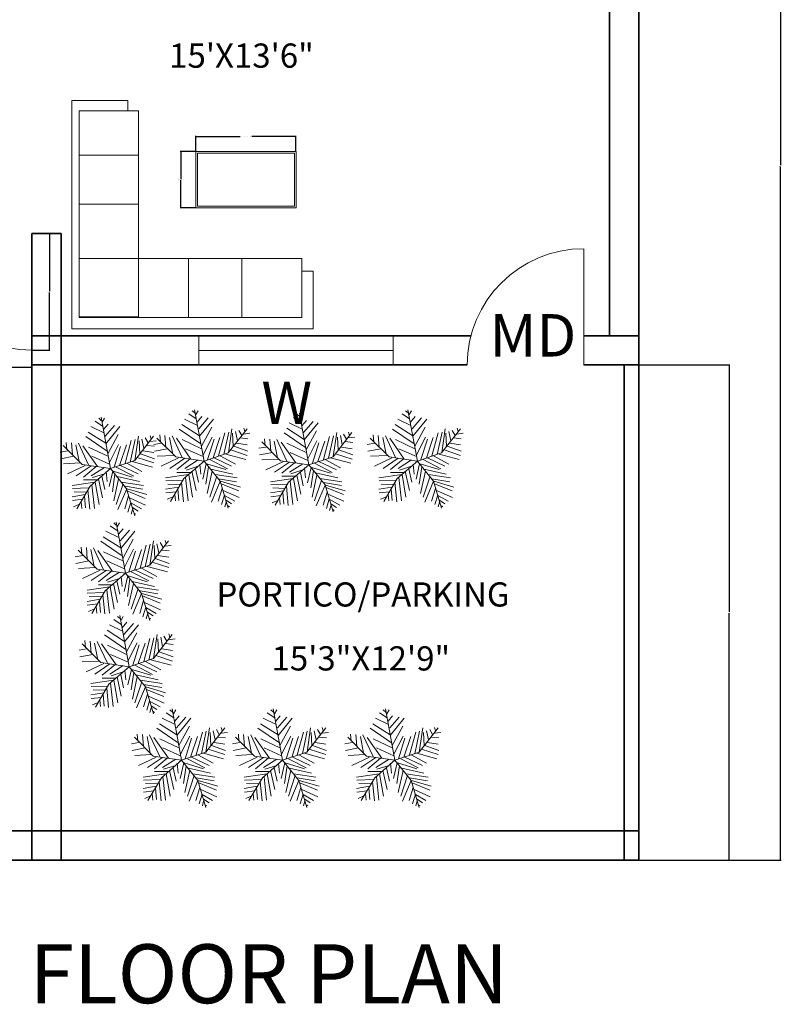
# Model space of a CAD drawing. Units: inches. Extents: x -26 to 788, y -42 to 505.
# Tile 4 of 9: x 116 to 352, y -42 to 262. Entities that reach past the tile are written whole.
import ezdxf

# ---------------------------------------------------------------- set-up
doc = ezdxf.new("R2010")
doc.units = ezdxf.units.IN
doc.header["$MEASUREMENT"] = 0
for name, color, linetype, lineweight in [('A-ANNO-DIMS', 2, 'Continuous', 18), ('A-ANNO-IDEN', 3, 'Continuous', 18), ('A-ANNO-TEXT', 7, 'Continuous', 25), ('A-AREA-IDEN', 7, 'Continuous', 18), ('A-DOOR', 3, 'Continuous', 18), ('A-FURN', 8, 'Continuous', 18), ('A-GLAZ', 4, 'Continuous', 18), ('A-WALL', 7, 'Continuous', 35), ('L-PLNT', 94, 'Continuous', 13)]:
    doc.layers.add(name, color=color, linetype=linetype, lineweight=lineweight)
doc.styles.get("Standard").update_dxf_attribs({"font": 'arial.ttf'})
doc.dimstyles.get("Standard").update_dxf_attribs({"dimtxt": 0.18, "dimasz": 0.18, "dimexe": 0.18, "dimexo": 0.0625, "dimgap": 0.09, "dimtad": 0, "dimtih": 1, "dimtoh": 1, "dimdec": 4, "dimzin": 0, "dimdsep": 46, "dimtxsty": 'Standard', "dimcen": 0.09, "dimadec": 0, "dimazin": 0, "dimtfac": 1, "dimtdec": 4, "dimtofl": 0, "dimtmove": 0, "dimatfit": 3, "dimfxl": 1, "dimtolj": 1, "dimtzin": 0, "dimarcsym": 0})

# ---------------------------------------------------------------- blocks, each defined once
blk = doc.blocks.new('*D8')
at = {"layer": 'A-ANNO-DIMS', "color": 0, "lineweight": -2, "transparency": 16777216}
for p, q in [((307.52, 431.12), (351.51, 431.12)), ((351.33, 430.94), (351.33, 216.8)), ((351.33, 2.3), (351.33, 216.44)), ((307.52, 2.12), (351.51, 2.12))]:
    blk.add_line(p, q, dxfattribs=at)
at = {"layer": 'A-ANNO-DIMS', "color": 0, "transparency": 16777216}
for points in [[(351.3, 430.94), (351.36, 430.94), (351.33, 431.12)], [(351.3, 2.3), (351.36, 2.3), (351.33, 2.12)]]:
    blk.add_solid(points, dxfattribs=at)
at = {"layer": 'Defpoints', "color": 0, "transparency": 16777216}
for p in [(307.45, 431.12), (307.45, 2.12), (351.33, 2.12)]:
    blk.add_point(p, dxfattribs=at)
at = {"layer": 'A-ANNO-DIMS', "color": 0, "transparency": 16777216, "insert": (351.33, 216.62), "char_height": 0.18, "attachment_point": 5}
blk.add_mtext('\\A1;429.0000', dxfattribs=at)
blk = doc.blocks.new('*U11')
for p, q in [((-258.7244, 1362.456), (-332.3336, 1421.4348)), ((0, 0), (-266.7, 1447.8)), ((-231.1146, 1315.2628), (-166.7002, 1421.4348)), ((-185.1152, 1008.5578), (-553.1612, 1185.4942)), ((-221.9198, 1197.3052), (-433.5526, 1338.8594)), ((-194.31, 1102.9442), (-65.4812, 1256.284)), ((-148.3106, 914.1968), (118.5418, 1220.9018)), ((-129.8956, 701.8528), (265.7602, 1185.4942)), ((-93.091, 489.5342), (-700.3796, 902.3858)), ((-129.8956, 713.6638), (-626.7704, 1032.1544)), ((-74.7014, 418.7444), (219.7608, 961.39)), ((685.8, 228.6), (1219.2, 914.4)), ((689.0258, 230.0224), (790.2448, 914.1968)), ((983.4626, 867.0036), (1066.2666, 725.4494)), ((1121.4862, 925.9824), (1149.0706, 831.6214)), ((-800.1, 114.3), (-1333.5, 647.7)), ((-1234.059, 536.7274), (-1252.4486, 737.2604)), ((-1105.2302, 725.4494), (-1077.6458, 395.1732)), ((-976.4268, 666.4706), (-884.4026, 194.6402)), ((-902.8176, 713.6638), (-617.5756, 100.2538)), ((-369.1382, 53.086), (-783.1836, 642.874)), ((-617.5756, 607.4918), (-74.7014, 347.98)), ((-28.6766, 171.0436), (228.9556, 678.2816)), ((100.1268, 41.275), (284.1498, 619.2774)), ((256.5654, 88.4682), (449.7832, 666.4706)), ((412.9786, 147.447), (587.8068, 796.2392)), ((560.197, 182.8292), (698.2206, 819.8358)), ((808.6344, 784.4282), (827.0494, 418.7444)), ((891.4384, 831.6214), (946.658, 572.1096)), ((1029.462, 654.685), (1241.0948, 631.0884)), ((1112.2914, 760.8316), (1296.3144, 784.4282)), ((-1206.4492, 501.3198), (-1418.082, 465.9376)), ((-1031.621, 347.98), (-1399.667, 277.1902)), ((-525.5514, 347.98), (-28.6766, 123.8504)), ((753.4148, 312.5978), (1222.6798, 159.2326)), ((845.439, 418.7444), (1241.0948, 277.1902)), ((919.0482, 501.3198), (1222.6798, 454.152)), ((-847.598, 159.2326), (-1326.0578, 135.636)), ((-718.7946, 88.4682), (-1215.644, -147.447)), ((-543.9664, 76.6572), (-967.2066, -206.4512)), ((0, 0), (-800.1, 114.3)), ((-405.9428, 53.086), (-764.794, -241.8334)), ((0, 0), (-571.5, -495.3)), ((-166.7002, 29.4894), (-543.9664, -206.4512)), ((0, 0), (685.8, 228.6)), ((0, 0), (457.2, -571.5)), ((164.5412, 41.275), (661.416, -218.2368)), ((284.1498, 88.4682), (781.0246, -147.447)), ((458.978, 147.447), (891.4384, -88.4682)), ((615.4166, 194.6402), (1185.8752, 41.275)), ((-166.7002, -147.447), (-507.1618, -253.619)), ((-240.3094, -218.2368), (-157.5054, -595.7062)), ((-120.7008, -88.4682), (-93.091, -371.5766)), ((63.3222, -76.6826), (-37.8714, -513.1308)), ((44.9326, -64.897), (615.4166, -241.8334)), ((127.7366, -159.258), (54.1274, -654.685)), ((192.151, -230.0224), (817.8292, -371.5766)), ((-442.7474, -383.3876), (-1086.8406, -477.7486)), ((-617.5756, -548.5384), (-1077.6458, -560.324)), ((-571.5, -495.3), (-952.5, -1143)), ((-387.5278, -324.4088), (-764.794, -324.4088)), ((-525.5514, -465.963), (-451.9422, -1126.5408)), ((-433.5526, -383.3876), (-323.1134, -1020.3688)), ((-341.5284, -289.0012), (-221.9198, -831.6214)), ((228.9556, -289.0012), (90.932, -914.1968)), ((357.759, -430.5554), (164.5412, -1020.3688)), ((311.7596, -383.3876), (937.4378, -477.7486)), ((412.9786, -501.3452), (919.0482, -583.9206)), ((-718.7946, -737.2604), (-1086.8406, -796.2392)), ((-681.9646, -666.496), (-1022.4262, -654.685)), ((-737.1842, -784.4536), (-709.5744, -1114.7298)), ((-635.9652, -607.5172), (-580.771, -1150.1374)), ((458.978, -572.1096), (210.5406, -1161.923)), ((514.1976, -772.6426), (403.7838, -1138.3264)), ((457.2, -571.5), (685.8, -1333.5)), ((468.1982, -572.1096), (1029.462, -737.2604)), ((486.5878, -642.8994), (983.4626, -843.4324)), ((541.8074, -831.6214), (992.6574, -1032.1544)), ((-783.1836, -867.029), (-1077.6458, -902.4112)), ((-875.2078, -1008.5832), (-1040.8412, -1079.3476)), ((-829.2084, -937.7934), (-810.7934, -1126.5408)), ((578.612, -961.39), (495.7826, -1232.7128)), ((578.612, -973.1756), (873.0488, -1138.3264)), ((624.6114, -1102.9442), (781.0246, -1209.1162)), ((624.6114, -1161.923), (587.8068, -1291.6916)), ((679.8056, -1268.095), (716.6102, -1291.6916))]:
    blk.add_line(p, q)
blk = doc.blocks.new('WIN-SLIDER-60')
for p, q in [((0, 9), (0, 0)), ((60, 9), (60, 0)), ((0, 4.5), (60, 4.5)), ((60, 4.5), (50.65, 4.5))]:
    blk.add_line(p, q)
blk = doc.blocks.new('DOOR-BEDROOM-36')
blk.add_line((36, 0), (36, 36))
blk.add_arc((36, 36), 36, 180, 270)
blk = doc.blocks.new('DOOR-ENTRY-36')
blk.add_line((36, 0), (36, 36))
blk.add_arc((36, 0), 36, 90, 179.8595)
blk = doc.blocks.new('SOFA-SECTIONAL')
for p, q in [((0, 17.98), (0, 70.62)), ((0, 70.62), (17.39, 70.62)), ((17.39, 70.62), (17.39, 67.34)), ((2.33, 53.68), (20.61, 53.68)), ((2.33, 38.52), (20.61, 38.52)), ((36.15, 21.72), (36.15, 3.64)), ((52.61, 21.72), (52.61, 3.64))]:
    blk.add_line(p, q)
for points in [[(2.33, 3.73), (20.67, 3.73), (20.67, 67.34), (2.33, 67.34)], [(2.32, 21.71), (71.08, 21.71), (71.08, 3.56), (2.32, 3.56)]]:
    blk.add_lwpolyline(points, close=True)
blk.add_lwpolyline([(71.08, 17.8), (74.64, 17.8), (74.64, 0), (0, 0), (0, 17.98)])
blk = doc.blocks.new('TABLE-COFFEE')
for points in [[(0, 17.36), (30.93, 17.36), (30.93, 0), (0, 0)], [(0.5, 16.86), (30.43, 16.86), (30.43, 0.5), (0.5, 0.5)]]:
    blk.add_lwpolyline(points, close=True)
blk = doc.blocks.new('*D35')
at = {"layer": 'A-ANNO-DIMS', "color": 0, "lineweight": -2, "transparency": 16777216}
for p, q in [((83.95, 159.65), (83.95, 154.13)), ((119.95, 159.65), (119.95, 154.13)), ((84.13, 154.31), (100.02, 154.31)), ((119.77, 154.31), (103.89, 154.31))]:
    blk.add_line(p, q, dxfattribs=at)
at = {"layer": 'A-ANNO-DIMS', "color": 0, "transparency": 16777216}
for points in [[(84.13, 154.34), (84.13, 154.28), (83.95, 154.31)], [(119.77, 154.34), (119.77, 154.28), (119.95, 154.31)]]:
    blk.add_solid(points, dxfattribs=at)
at = {"layer": 'Defpoints', "color": 0, "transparency": 16777216}
for p in [(83.95, 159.71), (119.95, 159.71), (119.95, 154.31)]:
    blk.add_point(p, dxfattribs=at)
at = {"layer": 'A-ANNO-DIMS', "color": 0, "transparency": 16777216, "insert": (101.95, 154.31), "char_height": 0.18, "attachment_point": 5}
blk.add_mtext('\\A1;BEDROOM DOOR 36.0000 TYP.', dxfattribs=at)
blk = doc.blocks.new('*D36')
at = {"layer": 'A-ANNO-DIMS', "color": 0, "lineweight": -2, "transparency": 16777216}
for p, q in [((120.02, 195.71), (125.53, 195.71)), ((125.35, 195.53), (125.35, 177.89)), ((125.35, 159.89), (125.35, 177.53)), ((120.02, 159.71), (125.53, 159.71))]:
    blk.add_line(p, q, dxfattribs=at)
at = {"layer": 'A-ANNO-DIMS', "color": 0, "transparency": 16777216}
for points in [[(125.32, 195.53), (125.38, 195.53), (125.35, 195.71)], [(125.32, 159.89), (125.38, 159.89), (125.35, 159.71)]]:
    blk.add_solid(points, dxfattribs=at)
at = {"layer": 'Defpoints', "color": 0, "transparency": 16777216}
for p in [(119.95, 195.71), (125.35, 195.71), (119.95, 159.71)]:
    blk.add_point(p, dxfattribs=at)
at = {"layer": 'A-ANNO-DIMS', "color": 0, "transparency": 16777216, "insert": (125.35, 177.71), "char_height": 0.18, "attachment_point": 5}
blk.add_mtext('\\A1;36.0000 TYP.', dxfattribs=at)
blk = doc.blocks.new('*D47')
at = {"layer": 'A-ANNO-DIMS', "color": 0, "lineweight": -2, "transparency": 16777216}
for p, q in [((170.63, 221.13), (170.63, 225.89)), ((170.81, 225.71), (184.28, 225.71)), ((201.38, 225.71), (187.92, 225.71)), ((201.56, 221.13), (201.56, 225.89))]:
    blk.add_line(p, q, dxfattribs=at)
at = {"layer": 'A-ANNO-DIMS', "color": 0, "transparency": 16777216}
for points in [[(170.81, 225.74), (170.81, 225.68), (170.63, 225.71)], [(201.38, 225.74), (201.38, 225.68), (201.56, 225.71)]]:
    blk.add_solid(points, dxfattribs=at)
at = {"layer": 'Defpoints', "color": 0, "transparency": 16777216}
for p in [(201.56, 225.71), (170.63, 221.07), (201.56, 221.07)]:
    blk.add_point(p, dxfattribs=at)
at = {"layer": 'A-ANNO-DIMS', "color": 0, "transparency": 16777216, "insert": (186.1, 225.71), "char_height": 0.18, "attachment_point": 5}
blk.add_mtext('\\A1;COFFEE TABLE 30.9297 TYP.', dxfattribs=at)
blk = doc.blocks.new('*D48')
at = {"layer": 'A-ANNO-DIMS', "color": 0, "lineweight": -2, "transparency": 16777216}
for p, q in [((170.57, 221.07), (165.82, 221.07)), ((166, 220.89), (166, 212.57)), ((166, 203.88), (166, 212.2)), ((170.57, 203.7), (165.82, 203.7))]:
    blk.add_line(p, q, dxfattribs=at)
at = {"layer": 'A-ANNO-DIMS', "color": 0, "transparency": 16777216}
for points in [[(165.97, 220.89), (166.03, 220.89), (166, 221.07)], [(165.97, 203.88), (166.03, 203.88), (166, 203.7)]]:
    blk.add_solid(points, dxfattribs=at)
at = {"layer": 'Defpoints', "color": 0, "transparency": 16777216}
for p in [(166, 221.07), (170.63, 221.07), (170.63, 203.7)]:
    blk.add_point(p, dxfattribs=at)
at = {"layer": 'A-ANNO-DIMS', "color": 0, "transparency": 16777216, "insert": (166, 212.39), "char_height": 0.18, "attachment_point": 5}
blk.add_mtext('\\A1;17.3631 TYP.', dxfattribs=at)
blk = doc.blocks.new('*D52')
at = {"layer": 'A-ANNO-DIMS', "color": 0, "lineweight": -2, "transparency": 16777216}
for p, q in [((307.52, 155.12), (335.58, 155.12)), ((335.4, 154.94), (335.4, 78.8)), ((335.4, 2.3), (335.4, 78.44)), ((307.52, 2.12), (335.58, 2.12))]:
    blk.add_line(p, q, dxfattribs=at)
at = {"layer": 'A-ANNO-DIMS', "color": 0, "transparency": 16777216}
for points in [[(335.37, 154.94), (335.43, 154.94), (335.4, 155.12)], [(335.37, 2.3), (335.43, 2.3), (335.4, 2.12)]]:
    blk.add_solid(points, dxfattribs=at)
at = {"layer": 'Defpoints', "color": 0, "transparency": 16777216}
for p in [(307.45, 155.12), (335.4, 155.12), (307.45, 2.12)]:
    blk.add_point(p, dxfattribs=at)
at = {"layer": 'A-ANNO-DIMS', "color": 0, "transparency": 16777216, "insert": (335.4, 78.62), "char_height": 0.18, "attachment_point": 5}
blk.add_mtext('\\A1;153.0000', dxfattribs=at)

msp = doc.modelspace()

# ---------------------------------------------------------------- linework, layer by layer
at = {"layer": 'A-WALL'}
for p, q in [((298.45497, 164.11777), (298.45497, 422.11777)), ((307.45497, 2.11777), (307.45497, 308.37421)), ((119.95497, 2.11777), (119.95497, 195.70898)), ((128.95497, 195.70898), (119.95497, 195.70898)), ((128.95497, 2.11777), (128.95497, 195.70898)), ((119.95497, 164.11777), (255.64361, 164.11777)), ((290.47756, 164.11777), (307.45497, 164.11777)), ((119.95497, 155.11777), (254.47767, 155.11777)), ((290.47756, 155.11777), (307.45497, 155.11777)), ((302.95497, 2.11777), (302.95497, 155.11777)), ((2.95497, 11.11777), (307.45497, 11.11777)), ((2.95497, 2.11777), (307.45497, 2.11777))]:
    msp.add_line(p, q, dxfattribs=at)

# ---------------------------------------------------------------- block references
at = {"layer": 'A-DOOR'}
for name, p in [('DOOR-BEDROOM-36', (83.955, 159.709)), ('DOOR-ENTRY-36', (254.478, 155.03))]:
    msp.add_blockref(name, p, dxfattribs=at)
at = {"layer": 'A-FURN'}
for name, p in [('SOFA-SECTIONAL', (132.246, 166.249)), ('TABLE-COFFEE', (170.635, 203.704))]:
    msp.add_blockref(name, p, dxfattribs=at)
at = {"layer": 'A-GLAZ'}
msp.add_blockref('WIN-SLIDER-60', (171.576, 155.082), dxfattribs=at)
at = {"layer": 'L-PLNT', "xscale": 0.0109273732196715, "yscale": 0.0109273732196715, "zscale": 0.0109273732196715}
for p in [(173.1455, 125.41083), (205.5306, 124.25531), (239.07231, 125.41083), (144.23022, 123.0998), (148.85667, 90.7453), (150.01327, 61.85734), (166.20583, 32.96939), (197.43431, 32.96939), (232.13263, 32.96939)]:
    msp.add_blockref('*U11', p, dxfattribs=at)

# ---------------------------------------------------------------- texts
at = {"layer": 'A-ANNO-IDEN'}
for s, height, p in [('MD', 13.093175, (261.37994, 157.71356)), ('W', 13.09317, (190.87154, 136.87714))]:
    msp.add_text(s, height=height, dxfattribs=at).set_placement(p)
at = {"layer": 'A-ANNO-TEXT'}
msp.add_text('GROUND FLOOR PLAN', height=18.2344212, dxfattribs=at).set_placement((9.22807, -42.14293))
at = {"layer": 'A-AREA-IDEN'}
for s, height, p in [('15\'X13\'6"', 7.483862, (162.36791, 246.95422)), ('PORTICO/PARKING', 7.4588445, (176.99189, 80.45125)), ('15\'3"X12\'9"', 7.4838625, (193.99632, 60.68919))]:
    msp.add_text(s, height=height, dxfattribs=at).set_placement(p)

# ---------------------------------------------------------------- dimensions: what is measured, and where the dimension line sits
at = {"layer": 'A-ANNO-DIMS'}
for base, p1, p2, override, picture, middle in [((351.33135, 2.11777), (307.45497, 431.11777), (307.45497, 2.11777), {"dimclrd": 0, "dimclre": 0, "dimclrt": 0}, '*D8', (351.33135, 216.61777)), ((335.40497, 155.11777), (307.45497, 2.11777), (307.45497, 155.11777), {"dimdec": 4, "dimlfac": 1, "dimrnd": 0, "dimzin": 0, "dimdsep": 46, "dimlunit": 2}, '*D52', (335.40497, 78.61777))]:
    dim = msp.add_linear_dim(base=base, p1=p1, p2=p2, angle=90, dimstyle='Standard', override=override, dxfattribs=at)
    dim.commit()
    dim.dimension.update_dxf_attribs({"geometry": picture, "text_midpoint": middle})
for base, p1, p2, text, picture, middle in [((201.56433, 225.70617), (170.63465, 221.06672), (201.56433, 221.06672), 'COFFEE TABLE <> TYP.', '*D47', (186.09949, 225.70617)), ((119.95497, 154.30898), (83.95497, 159.70898), (119.95497, 159.70898), 'BEDROOM DOOR <> TYP.', '*D35', (101.95497, 154.30898))]:
    dim = msp.add_linear_dim(base=base, p1=p1, p2=p2, text=text, dimstyle='Standard', override={"dimdec": 4, "dimlfac": 1, "dimrnd": 0, "dimzin": 0, "dimdsep": 46, "dimlunit": 2}, dxfattribs=at)
    dim.commit()
    dim.dimension.update_dxf_attribs({"geometry": picture, "text_midpoint": middle})
for base, p1, p2, picture, middle in [((165.9952, 221.06672), (170.63465, 203.70361), (170.63465, 221.06672), '*D48', (165.9952, 212.38516)), ((125.35497, 195.70898), (119.95497, 159.70898), (119.95497, 195.70898), '*D36', (125.35497, 177.70898))]:
    dim = msp.add_linear_dim(base=base, p1=p1, p2=p2, angle=90, text='<> TYP.', dimstyle='Standard', override={"dimdec": 4, "dimlfac": 1, "dimrnd": 0, "dimzin": 0, "dimdsep": 46, "dimlunit": 2}, dxfattribs=at)
    dim.commit()
    dim.dimension.update_dxf_attribs({"geometry": picture, "text_midpoint": middle})

doc.saveas('drawing.dxf')
